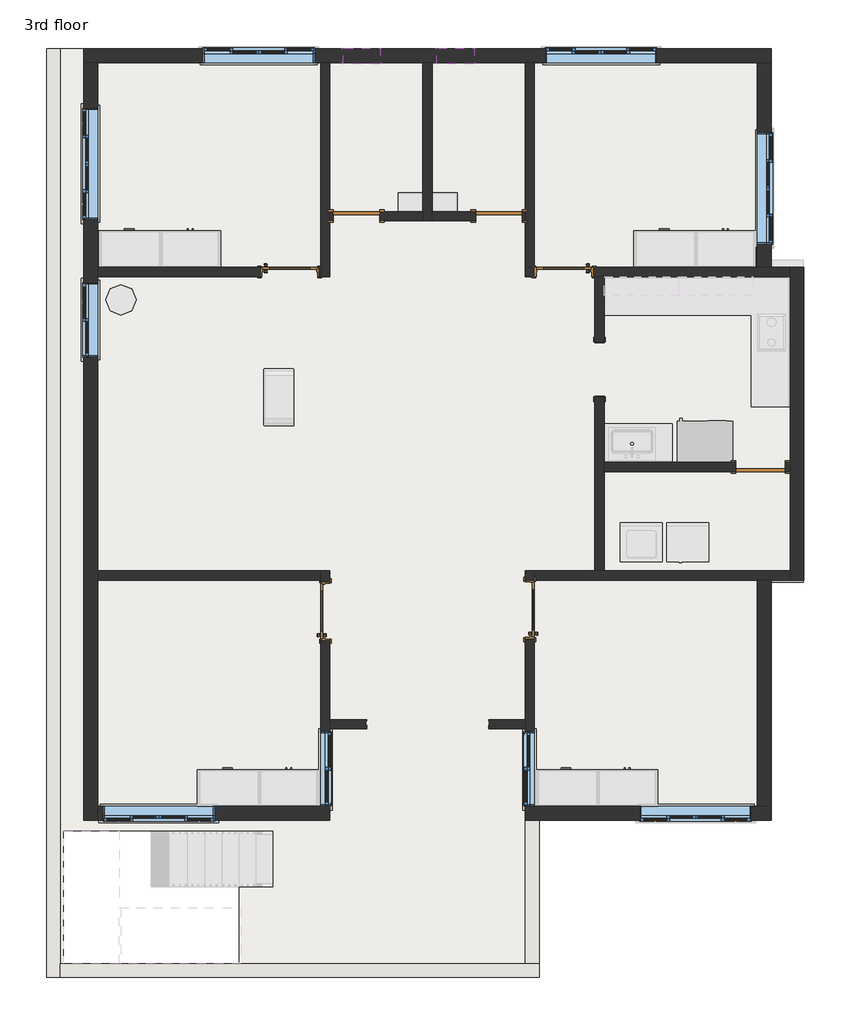
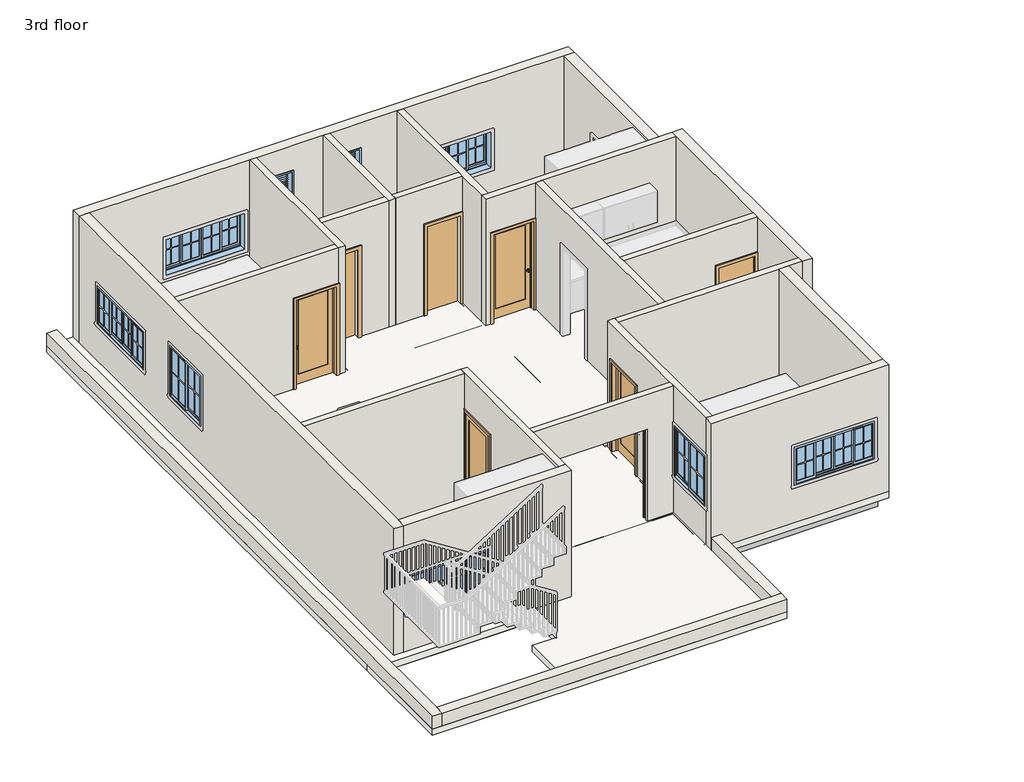
# One storey, part 1 of 4: 24 walls, 11 windows, 7 beams, 7 doors, 1 slab.
"""IFC4 building model written with IfcOpenShell, lengths in millimetres."""

from ifc_helpers import new_model, si_unit, frame, origin, place, context, project, spatial, polyline, outline, extrude, faceted_brep, transform, mapped, element, save
from components import door_010cc4d9, door_5a860750, door_e2b13fe9, door_a9addea7, door_bb092f7c, window_f2d8fef0, window_c1e3dfc0, window_49fe3060, window_58cce754

model = new_model("IFC4")

# Units and contexts
model_context = context("Model", 3, world=origin())
ifc_project = project(units=[si_unit("LENGTHUNIT", "METRE", prefix="MILLI")], contexts=[model_context])

# Site, building, storey
site = spatial("IfcSite", under=ifc_project)
building = spatial("IfcBuilding", under=site)
storey = spatial("IfcBuildingStorey", under=building, Name="3rd floor", Elevation=10210.8)

# Beams
placement = place(None, origin())
element("IfcBeam", 1, ObjectType="Concrete-Rectangular Beam", at=placement, inside=storey, context=model_context, shape_type="SweptSolid", body=[
    extrude(outline(polyline([(-1593.2124084, 1316.1961804), (-1364.6124084, 1316.1961804), (-1364.6124084, -2163.6038196), (-1593.2124084, -2163.6038196), (-1593.2124084, 1316.1961804)])), frame((0.0, 0.0, 9906.0), z_axis=(0.0, 0.0, 1.0), x_axis=(1.0, 0.0, 0.0)), (0.0, 0.0, 1.0), 304.8),
])
element("IfcBeam", 2, ObjectType="Concrete-Rectangular Beam", at=placement, inside=storey, context=model_context, shape_type="Brep", body=[
    faceted_brep([(-1593.2124084, -2201.7038196, 10210.8), (-5212.7124084, -2201.7038196, 10210.8), (-5441.3124084, -2201.7038196, 10210.8), (-5441.3124084, -2239.8038196, 10210.8), (-5174.6124084, -2239.8038196, 10210.8), (-5174.6124084, -2430.3038196, 10210.8), (-1593.2124084, -2430.3038196, 10210.8), (-1593.2124084, -2201.7038196, 9906.0), (-5212.7124084, -2201.7038196, 9906.0), (-5441.3124084, -2201.7038196, 9906.0), (-1593.2124084, -2430.3038196, 9906.0), (-5174.6124084, -2430.3038196, 9906.0), (-5174.6124084, -2239.8038196, 9906.0), (-5441.3124084, -2239.8038196, 9906.0)], [[[0, 1, 2, 3, 4, 5, 6]], [[0, 7, 8, 9, 2, 1]], [[9, 8, 7, 10, 11, 12, 13]], [[10, 6, 5, 11]], [[7, 0, 6, 10]], [[2, 9, 13, 3]], [[12, 4, 3, 13]], [[4, 12, 11, 5]]]),
])
element("IfcBeam", 3, ObjectType="Concrete-Rectangular Beam", at=placement, inside=storey, context=model_context, shape_type="Brep", body=[
    faceted_brep([(-8756.0124084, -2468.4038196, 10210.8), (-8756.0124084, -2239.8038196, 10210.8), (-8794.1124084, -2239.8038196, 10210.8), (-12413.6124084, -2239.8038196, 10210.8), (-12413.6124084, -2468.4038196, 10210.8), (-8756.0124084, -2239.8038196, 9906.0), (-8794.1124084, -2239.8038196, 9906.0), (-12413.6124084, -2239.8038196, 9906.0), (-8756.0124084, -2468.4038196, 9906.0), (-12413.6124084, -2468.4038196, 9906.0)], [[[0, 1, 2, 3, 4]], [[1, 5, 6, 7, 3, 2]], [[5, 8, 9, 7, 6]], [[8, 0, 4, 9]], [[1, 0, 8, 5]], [[4, 3, 7, 9]]]),
])
element("IfcBeam", 4, ObjectType="Concrete-Rectangular Beam", at=placement, inside=storey, context=model_context, shape_type="SweptSolid", body=[
    extrude(outline(polyline([(-12642.2124084, 9875.9961804), (-12413.6124084, 9875.9961804), (-12413.6124084, 6751.7961804), (-12642.2124084, 6751.7961804), (-12642.2124084, 9875.9961804)])), frame((0.0, 0.0, 9906.0), z_axis=(0.0, 0.0, 1.0), x_axis=(1.0, 0.0, 0.0)), (0.0, 0.0, 1.0), 304.8),
    extrude(outline(polyline([(-12413.6124084, -2163.6038196), (-12642.2124084, -2163.6038196), (-12642.2124084, 1392.3961804), (-12413.6124084, 1392.3961804), (-12413.6124084, -2163.6038196)])), frame((0.0, 0.0, 9906.0), z_axis=(0.0, 0.0, 1.0), x_axis=(1.0, 0.0, 0.0)), (0.0, 0.0, 1.0), 304.8),
    extrude(outline(polyline([(-12413.6124084, 1697.1961804), (-12642.2124084, 1697.1961804), (-12642.2124084, 6446.9961804), (-12413.6124084, 6446.9961804), (-12413.6124084, 1697.1961804)])), frame((0.0, 0.0, 9906.0), z_axis=(0.0, 0.0, 1.0), x_axis=(1.0, 0.0, 0.0)), (0.0, 0.0, 1.0), 304.8),
])
element("IfcBeam", 5, ObjectType="Concrete-Rectangular Beam", at=placement, inside=storey, context=model_context, shape_type="Brep", body=[
    faceted_brep([(-843.9124084, 1659.0961804, 10210.8), (-843.9124084, 1430.4961804, 10210.8), (-843.9124084, 1430.4961804, 9906.0), (-843.9124084, 1659.0961804, 9906.0), (-5098.4124084, 1659.0961804, 10210.8), (-5098.4124084, 1468.5961804, 10210.8), (-5403.2124084, 1468.5961804, 10210.8), (-5403.2124084, 1659.0961804, 10210.8), (-5441.3124084, 1659.0961804, 10210.8), (-8565.5124084, 1659.0961804, 10210.8), (-8603.6124084, 1659.0961804, 10210.8), (-8603.6124084, 1468.5961804, 10210.8), (-8908.4124084, 1468.5961804, 10210.8), (-8908.4124084, 1659.0961804, 10210.8), (-12413.6124084, 1659.0961804, 10210.8), (-12413.6124084, 1430.4961804, 10210.8), (-8794.1124084, 1430.4961804, 10210.8), (-8565.5124084, 1430.4961804, 10210.8), (-5441.3124084, 1430.4961804, 10210.8), (-5212.7124084, 1430.4961804, 10210.8), (-1593.2124084, 1430.4961804, 10210.8), (-1593.2124084, 1620.9961804, 10210.8), (-1364.6124084, 1620.9961804, 10210.8), (-1364.6124084, 1430.4961804, 10210.8), (-1364.6124084, 1430.4961804, 9906.0), (-1364.6124084, 1620.9961804, 9906.0), (-1593.2124084, 1620.9961804, 9906.0), (-1593.2124084, 1430.4961804, 9906.0), (-5212.7124084, 1430.4961804, 9906.0), (-5441.3124084, 1430.4961804, 9906.0), (-8565.5124084, 1430.4961804, 9906.0), (-8794.1124084, 1430.4961804, 9906.0), (-12413.6124084, 1430.4961804, 9906.0), (-12413.6124084, 1659.0961804, 9906.0), (-8908.4124084, 1659.0961804, 9906.0), (-8908.4124084, 1468.5961804, 9906.0), (-8603.6124084, 1468.5961804, 9906.0), (-8603.6124084, 1659.0961804, 9906.0), (-8565.5124084, 1659.0961804, 9906.0), (-5441.3124084, 1659.0961804, 9906.0), (-5403.2124084, 1659.0961804, 9906.0), (-5403.2124084, 1468.5961804, 9906.0), (-5098.4124084, 1468.5961804, 9906.0), (-5098.4124084, 1659.0961804, 9906.0)], [[[0, 1, 2, 3]], [[1, 0, 4, 5, 6, 7, 8, 9, 10, 11, 12, 13, 14, 15, 16, 17, 18, 19, 20, 21, 22, 23]], [[2, 1, 23, 24]], [[3, 2, 24, 25, 26, 27, 28, 29, 30, 31, 32, 33, 34, 35, 36, 37, 38, 39, 40, 41, 42, 43]], [[0, 3, 43, 4]], [[15, 14, 33, 32]], [[23, 22, 25, 24]], [[21, 20, 27, 26]], [[22, 21, 26, 25]], [[15, 32, 31, 30, 29, 28, 27, 20, 19, 18, 17, 16]], [[11, 10, 37, 36]], [[12, 11, 36, 35]], [[13, 12, 35, 34]], [[33, 14, 13, 34]], [[42, 5, 4, 43]], [[5, 42, 41, 6]], [[6, 41, 40, 7]], [[37, 10, 9, 8, 7, 40, 39, 38]]]),
])
element("IfcBeam", 6, ObjectType="Concrete-Rectangular Beam", at=placement, inside=storey, context=model_context, shape_type="Brep", body=[
    faceted_brep([(-8794.1124084, -2239.8038196, 10210.8), (-8756.0124084, -2239.8038196, 10210.8), (-8565.5124084, -2239.8038196, 10210.8), (-8565.5124084, -1007.9038196, 10210.8), (-8565.5124084, -779.3038196, 10210.8), (-8565.5124084, 1430.4961804, 10210.8), (-8794.1124084, 1430.4961804, 10210.8), (-8794.1124084, -2239.8038196, 9906.0), (-8794.1124084, 1430.4961804, 9906.0), (-8565.5124084, -2239.8038196, 9906.0), (-8756.0124084, -2239.8038196, 9906.0), (-8565.5124084, 1430.4961804, 9906.0), (-8565.5124084, -779.3038196, 9906.0), (-8565.5124084, -1007.9038196, 9906.0)], [[[0, 1, 2, 3, 4, 5, 6]], [[7, 0, 6, 8]], [[9, 10, 7, 8, 11, 12, 13]], [[11, 5, 4, 3, 2, 9, 13, 12]], [[2, 1, 0, 7, 10, 9]], [[5, 11, 8, 6]]]),
    faceted_brep([(-8794.1124084, 9914.0961804, 10210.8), (-8565.5124084, 9914.0961804, 10210.8), (-8565.5124084, 9914.0961804, 9906.0), (-8794.1124084, 9914.0961804, 9906.0), (-8794.1124084, 6713.6961804, 10210.8), (-8794.1124084, 6713.6961804, 9906.0), (-8756.0124084, 6713.6961804, 9906.0), (-8756.0124084, 6713.6961804, 10210.8), (-8756.0124084, 6751.7961804, 10210.8), (-8565.5124084, 6751.7961804, 10210.8), (-8565.5124084, 7323.2961804, 10210.8), (-8565.5124084, 7551.8961804, 10210.8), (-8565.5124084, 7551.8961804, 9906.0), (-8565.5124084, 7323.2961804, 9906.0), (-8565.5124084, 6751.7961804, 9906.0), (-8756.0124084, 6751.7961804, 9906.0)], [[[0, 1, 2, 3]], [[4, 5, 6, 7]], [[1, 0, 4, 7, 8, 9, 10, 11]], [[3, 2, 12, 13, 14, 15, 6, 5]], [[0, 3, 5, 4]], [[2, 1, 11, 10, 9, 14, 13, 12]], [[7, 6, 15, 8]], [[9, 8, 15, 14]]]),
    faceted_brep([(-8794.1124084, 6485.0961804, 9906.0), (-8794.1124084, 6485.0961804, 10210.8), (-8756.0124084, 6485.0961804, 10210.8), (-8756.0124084, 6485.0961804, 9906.0), (-8565.5124084, 1659.0961804, 9906.0), (-8565.5124084, 1659.0961804, 10210.8), (-8603.6124084, 1659.0961804, 10210.8), (-8603.6124084, 1659.0961804, 9906.0), (-8565.5124084, 6446.9961804, 9906.0), (-8565.5124084, 6446.9961804, 10210.8), (-8794.1124084, 1697.1961804, 10210.8), (-8603.6124084, 1697.1961804, 10210.8), (-8756.0124084, 6446.9961804, 10210.8), (-8794.1124084, 1697.1961804, 9906.0), (-8603.6124084, 1697.1961804, 9906.0), (-8756.0124084, 6446.9961804, 9906.0)], [[[0, 1, 2, 3]], [[4, 5, 6, 7]], [[5, 4, 8, 9]], [[2, 1, 10, 11, 6, 5, 9, 12]], [[1, 0, 13, 10]], [[8, 4, 7, 14, 13, 0, 3, 15]], [[9, 8, 15, 12]], [[3, 2, 12, 15]], [[14, 11, 10, 13]], [[11, 14, 7, 6]]]),
])
element("IfcBeam", 7, ObjectType="Concrete-Rectangular Beam", at=placement, inside=storey, context=model_context, shape_type="SweptSolid", body=[
    extrude(outline(polyline([(-5441.3124084, -779.3038196), (-5441.3124084, -1007.9038196), (-8565.5124084, -1007.9038196), (-8565.5124084, -779.3038196), (-5441.3124084, -779.3038196)])), frame((0.0, 0.0, 9906.0), z_axis=(0.0, 0.0, 1.0), x_axis=(1.0, 0.0, 0.0)), (0.0, 0.0, 1.0), 304.8),
])

# Doors
door_shape = door_010cc4d9(model_context)
element("IfcDoor", 8, ObjectType="Door-Interior-Single-1_Panel-Wood : 36\" x 84\"", at=placement, inside=storey, context=model_context, shape_type="MappedRepresentation", body=[
    mapped(door_shape, transform((-9264.0124084, 6526.3711804, 10210.8), x_axis=(1.0, 0.0, 0.0), y_axis=(0.0, 1.0, 0.0), z_axis=(0.0, 0.0, 1.0))),
])
element("IfcDoor", 9, ObjectType="Door-Interior-Single-1_Panel-Wood : 36\" x 84\"", at=placement, inside=storey, context=model_context, shape_type="MappedRepresentation", body=[
    mapped(door_shape, transform((-8682.9874084, 960.5961804, 10210.8), x_axis=(0.0, 1.0, 0.0), y_axis=(-1.0, 0.0, 0.0), z_axis=(0.0, 0.0, 1.0))),
])
door_2_shape = door_5a860750(model_context)
element("IfcDoor", 10, ObjectType="Door-Interior-Single-1_Panel-Wood : 36\" x 84\"", at=placement, inside=storey, context=model_context, shape_type="MappedRepresentation", body=[
    mapped(door_2_shape, transform((-4768.2124084, 6526.3711804, 10210.8), x_axis=(-1.0, 0.0, 0.0), y_axis=(0.0, -1.0, 0.0), z_axis=(0.0, 0.0, 1.0))),
])
element("IfcDoor", 11, ObjectType="Door-Interior-Single-1_Panel-Wood : 36\" x 84\"", at=placement, inside=storey, context=model_context, shape_type="MappedRepresentation", body=[
    mapped(door_2_shape, transform((-5323.8374084, 985.9961804, 10210.8), x_axis=(0.0, 1.0, 0.0), y_axis=(-1.0, 0.0, 0.0), z_axis=(0.0, 0.0, 1.0))),
])
door_3_shape = door_e2b13fe9(model_context)
element("IfcDoor", 12, ObjectType="Single-Flush : 30\" x 84\"", at=placement, inside=storey, context=model_context, shape_type="MappedRepresentation", body=[
    mapped(door_3_shape, transform((-8171.8124084, 7437.5961804, 10210.8), x_axis=(-1.0, 0.0, 0.0), y_axis=(0.0, -1.0, 0.0), z_axis=(0.0, 0.0, 1.0))),
])
door_4_shape = door_a9addea7(model_context)
element("IfcDoor", 13, ObjectType="Single-Flush : 30\" x 84\"", at=placement, inside=storey, context=model_context, shape_type="MappedRepresentation", body=[
    mapped(door_4_shape, transform((-5835.0124084, 7437.5961804, 10210.8), x_axis=(1.0, 0.0, 0.0), y_axis=(0.0, 1.0, 0.0), z_axis=(0.0, 0.0, 1.0))),
])
door_5_shape = door_bb092f7c(model_context)
element("IfcDoor", 14, ObjectType="Single-Flush : 32\" x 84\"", at=placement, inside=storey, context=model_context, shape_type="MappedRepresentation", body=[
    mapped(door_5_shape, transform((-1542.4124084, 3322.7961804, 10210.8), x_axis=(1.0, 0.0, 0.0), y_axis=(0.0, 1.0, 0.0), z_axis=(0.0, 0.0, 1.0))),
])

# Slab
element("IfcSlab", 15, ObjectType="Generic - 6\"", at=placement, inside=storey, context=model_context, shape_type="SweptSolid", body=[
    extrude(outline(polyline([(-1364.6124084, 10180.7961804), (-1364.6124084, 6599.3961804), (-831.2124084, 6599.3961804), (-831.2124084, 1468.5961804), (-1364.6124084, 1468.5961804), (-1364.6124084, -2468.4038196), (-5174.6124084, -2468.4038196), (-5174.6124084, -5046.5038196), (-13251.8124084, -5046.5038196), (-13251.8124084, -2468.4038196), (-13251.8124084, 10180.7961804), (-1364.6124084, 10180.7961804)]), holes=[polyline([(-9543.8120641, -3536.9669819), (-9543.8120641, -2647.9669819), (-12972.8120641, -2647.9669819), (-12972.8120641, -4817.9038196), (-10102.6120641, -4817.9038196), (-10102.6120641, -3536.9669819), (-9543.8120641, -3536.9669819)])]), frame((0.0, 0.0, 10058.4), z_axis=(0.0, 0.0, 1.0), x_axis=(1.0, 0.0, 0.0)), (0.0, 0.0, 1.0), 152.4),
])

# Walls
element("IfcWall", 16, ObjectType="Generic - 6\"", at=placement, inside=storey, context=model_context, shape_type="Brep", body=[
    faceted_brep([(-8756.0124084, 9952.1961804, 10210.8), (-8756.0124084, 6599.3961804, 10210.8), (-8756.0124084, 6446.9961804, 10210.8), (-8756.0124084, 6446.9961804, 13258.8), (-8756.0124084, 6599.3961804, 13258.8), (-8756.0124084, 9952.1961804, 13258.8), (-8603.6124084, 9952.1961804, 10210.8), (-8603.6124084, 9952.1961804, 13258.8), (-8603.6124084, 7513.7961804, 13258.8), (-8603.6124084, 7361.3961804, 13258.8), (-8603.6124084, 6446.9961804, 13258.8), (-8603.6124084, 6446.9961804, 10210.8), (-8603.6124084, 7361.3961804, 10210.8), (-8603.6124084, 7513.7961804, 10210.8)], [[[0, 1, 2, 3, 4, 5]], [[6, 7, 8, 9, 10, 11, 12, 13]], [[2, 1, 0, 6, 13, 12, 11]], [[0, 5, 7, 6]], [[3, 2, 11, 10]], [[5, 4, 3, 10, 9, 8, 7]]]),
])
element("IfcWall", 17, ObjectType="Generic - 6\"", at=placement, inside=storey, context=model_context, shape_type="SweptSolid", body=[
    extrude(outline(polyline([(10210.8, -8756.0124084), (13258.8, -8756.0124084), (13258.8, -12413.6124084), (10210.8, -12413.6124084), (10210.8, -9746.6124084), (12369.8, -9746.6124084), (12369.8, -8781.4124084), (10210.8, -8781.4124084), (10210.8, -8756.0124084)])), frame((0.0, 6446.9961804, 0.0), z_axis=(0.0, 1.0, 0.0), x_axis=(0.0, 0.0, 1.0)), (0.0, 0.0, 1.0), 152.4),
])
element("IfcWall", 18, ObjectType="Generic - 6\"", at=placement, inside=storey, context=model_context, shape_type="Brep", body=[
    faceted_brep([(-7079.6124084, 9952.1961804, 10210.8), (-7079.6124084, 7513.7961804, 10210.8), (-7079.6124084, 7361.3961804, 10210.8), (-7079.6124084, 7361.3961804, 13258.8), (-7079.6124084, 7513.7961804, 13258.8), (-7079.6124084, 9952.1961804, 13258.8), (-6927.2124084, 9952.1961804, 10210.8), (-6927.2124084, 9952.1961804, 13258.8), (-6927.2124084, 7513.7961804, 13258.8), (-6927.2124084, 7361.3961804, 13258.8), (-6927.2124084, 7361.3961804, 10210.8), (-6927.2124084, 7513.7961804, 10210.8)], [[[0, 1, 2, 3, 4, 5]], [[6, 7, 8, 9, 10, 11]], [[2, 1, 0, 6, 11, 10]], [[0, 5, 7, 6]], [[3, 2, 10, 9]], [[5, 4, 3, 9, 8, 7]]]),
])
element("IfcWall", 19, ObjectType="Generic - 6\"", at=placement, inside=storey, context=model_context, shape_type="SweptSolid", body=[
    extrude(outline(polyline([(10210.8, -7079.6124084), (13258.8, -7079.6124084), (13258.8, -8603.6124084), (10210.8, -8603.6124084), (10210.8, -8552.8124084), (12344.4, -8552.8124084), (12344.4, -7790.8124084), (10210.8, -7790.8124084), (10210.8, -7079.6124084)])), frame((0.0, 7361.3961804, 0.0), z_axis=(0.0, 1.0, 0.0), x_axis=(0.0, 0.0, 1.0)), (0.0, 0.0, 1.0), 152.4),
])
element("IfcWall", 20, ObjectType="Generic - 6\"", at=placement, inside=storey, context=model_context, shape_type="SweptSolid", body=[
    extrude(outline(polyline([(13258.8, -6927.2124084), (10210.8, -6927.2124084), (10210.8, -6216.0124084), (12344.4, -6216.0124084), (12344.4, -5454.0124084), (10210.8, -5454.0124084), (10210.8, -5403.2124084), (13258.8, -5403.2124084), (13258.8, -6927.2124084)])), frame((0.0, 7361.3961804, 0.0), z_axis=(0.0, 1.0, 0.0), x_axis=(0.0, 0.0, 1.0)), (0.0, 0.0, 1.0), 152.4),
])
element("IfcWall", 21, ObjectType="Generic - 6\"", at=placement, inside=storey, context=model_context, shape_type="Brep", body=[
    faceted_brep([(-5250.8124084, 6599.3961804, 10210.8), (-5250.8124084, 9952.1961804, 10210.8), (-5250.8124084, 9952.1961804, 13258.8), (-5250.8124084, 6599.3961804, 13258.8), (-5403.2124084, 6599.3961804, 10210.8), (-5403.2124084, 6599.3961804, 13258.8), (-5403.2124084, 7361.3961804, 13258.8), (-5403.2124084, 7513.7961804, 13258.8), (-5403.2124084, 9952.1961804, 13258.8), (-5403.2124084, 9952.1961804, 10210.8), (-5403.2124084, 7513.7961804, 10210.8), (-5403.2124084, 7361.3961804, 10210.8)], [[[0, 1, 2, 3]], [[4, 5, 6, 7, 8, 9, 10, 11]], [[1, 0, 4, 11, 10, 9]], [[2, 1, 9, 8]], [[0, 3, 5, 4]], [[3, 2, 8, 7, 6, 5]]]),
])
element("IfcWall", 22, ObjectType="Generic - 6\"", at=placement, inside=storey, context=model_context, shape_type="Brep", body=[
    faceted_brep([(-5403.2124084, 6599.3961804, 10210.8), (-5403.2124084, 6599.3961804, 13258.8), (-5250.8124084, 6599.3961804, 13258.8), (-1593.2124084, 6599.3961804, 13258.8), (-1364.6124084, 6599.3961804, 13258.8), (-1059.8124084, 6599.3961804, 13258.8), (-1059.8124084, 6599.3961804, 10210.8), (-1364.6124084, 6599.3961804, 10210.8), (-1593.2124084, 6599.3961804, 10210.8), (-4285.6124084, 6599.3961804, 10210.8), (-4285.6124084, 6599.3961804, 12369.8), (-5250.8124084, 6599.3961804, 12369.8), (-5250.8124084, 6599.3961804, 10210.8), (-1059.8124084, 6446.9961804, 13258.8), (-4107.8124084, 6446.9961804, 13258.8), (-4260.2124084, 6446.9961804, 13258.8), (-5403.2124084, 6446.9961804, 13258.8), (-5403.2124084, 6446.9961804, 10210.8), (-5250.8124084, 6446.9961804, 10210.8), (-5250.8124084, 6446.9961804, 12369.8), (-4285.6124084, 6446.9961804, 12369.8), (-4285.6124084, 6446.9961804, 10210.8), (-4260.2124084, 6446.9961804, 10210.8), (-4107.8124084, 6446.9961804, 10210.8), (-1059.8124084, 6446.9961804, 10210.8)], [[[0, 1, 2, 3, 4, 5, 6, 7, 8, 9, 10, 11, 12]], [[13, 14, 15, 16, 17, 18, 19, 20, 21, 22, 23, 24]], [[17, 0, 12, 18]], [[6, 24, 23, 22, 21, 9, 8, 7]], [[1, 0, 17, 16]], [[6, 5, 13, 24]], [[11, 19, 18, 12]], [[19, 11, 10, 20]], [[20, 10, 9, 21]], [[16, 15, 14, 13, 5, 4, 3, 2, 1]]]),
])
element("IfcWall", 23, ObjectType="Generic - 6\"", at=placement, inside=storey, context=model_context, shape_type="SweptSolid", body=[
    extrude(outline(polyline([(-8756.0124084, 1468.5961804), (-12413.6124084, 1468.5961804), (-12413.6124084, 1620.9961804), (-8756.0124084, 1620.9961804), (-8756.0124084, 1468.5961804)])), frame((0.0, 0.0, 10210.8), z_axis=(0.0, 0.0, 1.0), x_axis=(1.0, 0.0, 0.0)), (0.0, 0.0, 1.0), 3048.0),
])
element("IfcWall", 24, ObjectType="Generic - 6\"", at=placement, inside=storey, context=model_context, shape_type="Brep", body=[
    faceted_brep([(-5403.2124084, -2239.8038196, 10210.8), (-5403.2124084, -2239.8038196, 13258.8), (-5403.2124084, -969.8038196, 13258.8), (-5403.2124084, -817.4038196, 13258.8), (-5403.2124084, 1620.9961804, 13258.8), (-5403.2124084, 1620.9961804, 10210.8), (-5403.2124084, 1468.5961804, 10210.8), (-5403.2124084, 1468.5961804, 12369.8), (-5403.2124084, 503.3961804, 12369.8), (-5403.2124084, 503.3961804, 10210.8), (-5403.2124084, -817.4038196, 10210.8), (-5403.2124084, -969.8038196, 10210.8), (-5403.2124084, -1014.2538196, 11125.2), (-5403.2124084, -1014.2538196, 12344.4), (-5403.2124084, -2233.4538196, 12344.4), (-5403.2124084, -2233.4538196, 11125.2), (-5250.8124084, -2239.8038196, 13258.8), (-5250.8124084, -2239.8038196, 10210.8), (-5250.8124084, 503.3961804, 10210.8), (-5250.8124084, 503.3961804, 12369.8), (-5250.8124084, 1468.5961804, 12369.8), (-5250.8124084, 1468.5961804, 10210.8), (-5250.8124084, 1620.9961804, 10210.8), (-5250.8124084, 1620.9961804, 13258.8), (-5250.8124084, 1468.5961804, 13258.8), (-5250.8124084, -1014.2538196, 12344.4), (-5250.8124084, -1014.2538196, 11125.2), (-5250.8124084, -2233.4538196, 11125.2), (-5250.8124084, -2233.4538196, 12344.4)], [[[0, 1, 2, 3, 4, 5, 6, 7, 8, 9, 10, 11], [12, 13, 14, 15]], [[16, 17, 18, 19, 20, 21, 22, 23, 24], [25, 26, 27, 28]], [[17, 0, 11, 10, 9, 18]], [[5, 22, 21, 6]], [[1, 0, 17, 16]], [[5, 4, 23, 22]], [[20, 7, 6, 21]], [[7, 20, 19, 8]], [[8, 19, 18, 9]], [[25, 13, 12, 26]], [[26, 12, 15, 27]], [[27, 15, 14, 28]], [[13, 25, 28, 14]], [[4, 3, 2, 1, 16, 24, 23]]]),
])
element("IfcWall", 25, ObjectType="Generic - 6\"", at=placement, inside=storey, context=model_context, shape_type="Brep", body=[
    faceted_brep([(-8756.0124084, 1620.9961804, 10210.8), (-8756.0124084, 1468.5961804, 10210.8), (-8756.0124084, 1443.1961804, 10210.8), (-8756.0124084, 1443.1961804, 12369.8), (-8756.0124084, 477.9961804, 12369.8), (-8756.0124084, 477.9961804, 10210.8), (-8756.0124084, -2239.8038196, 10210.8), (-8756.0124084, -2239.8038196, 13258.8), (-8756.0124084, 1468.5961804, 13258.8), (-8756.0124084, 1620.9961804, 13258.8), (-8756.0124084, -2233.4538196, 12344.4), (-8756.0124084, -2233.4538196, 11125.2), (-8756.0124084, -1014.2538196, 11125.2), (-8756.0124084, -1014.2538196, 12344.4), (-8603.6124084, 1443.1961804, 10210.8), (-8603.6124084, 1620.9961804, 10210.8), (-8603.6124084, 1620.9961804, 13258.8), (-8603.6124084, -817.4038196, 13258.8), (-8603.6124084, -969.8038196, 13258.8), (-8603.6124084, -2239.8038196, 13258.8), (-8603.6124084, -2239.8038196, 10210.8), (-8603.6124084, -969.8038196, 10210.8), (-8603.6124084, -817.4038196, 10210.8), (-8603.6124084, 477.9961804, 10210.8), (-8603.6124084, 477.9961804, 12369.8), (-8603.6124084, 1443.1961804, 12369.8), (-8603.6124084, -2233.4538196, 11125.2), (-8603.6124084, -2233.4538196, 12344.4), (-8603.6124084, -1014.2538196, 12344.4), (-8603.6124084, -1014.2538196, 11125.2)], [[[0, 1, 2, 3, 4, 5, 6, 7, 8, 9], [10, 11, 12, 13]], [[14, 15, 16, 17, 18, 19, 20, 21, 22, 23, 24, 25], [26, 27, 28, 29]], [[6, 5, 23, 22, 21, 20]], [[2, 1, 0, 15, 14]], [[25, 3, 2, 14]], [[3, 25, 24, 4]], [[4, 24, 23, 5]], [[0, 9, 16, 15]], [[10, 27, 26, 11]], [[11, 26, 29, 12]], [[12, 29, 28, 13]], [[27, 10, 13, 28]], [[9, 8, 7, 19, 18, 17, 16]], [[7, 6, 20, 19]]]),
])
element("IfcWall", 26, ObjectType="Generic - 6\"", at=placement, inside=storey, context=model_context, shape_type="Brep", body=[
    faceted_brep([(-4260.2124084, 6446.9961804, 13258.8), (-4260.2124084, 6446.9961804, 10210.8), (-4260.2124084, 5380.1961804, 10210.8), (-4260.2124084, 5380.1961804, 12344.4), (-4260.2124084, 4465.7961804, 12344.4), (-4260.2124084, 4465.7961804, 10210.8), (-4260.2124084, 1620.9961804, 10210.8), (-4260.2124084, 1620.9961804, 13258.8), (-4107.8124084, 6446.9961804, 10210.8), (-4107.8124084, 6446.9961804, 13258.8), (-4107.8124084, 3398.9961804, 13258.8), (-4107.8124084, 3246.5961804, 13258.8), (-4107.8124084, 1620.9961804, 13258.8), (-4107.8124084, 1620.9961804, 10210.8), (-4107.8124084, 3246.5961804, 10210.8), (-4107.8124084, 3398.9961804, 10210.8), (-4107.8124084, 4465.7961804, 10210.8), (-4107.8124084, 4465.7961804, 12344.4), (-4107.8124084, 5380.1961804, 12344.4), (-4107.8124084, 5380.1961804, 10210.8)], [[[0, 1, 2, 3, 4, 5, 6, 7]], [[8, 9, 10, 11, 12, 13, 14, 15, 16, 17, 18, 19]], [[1, 8, 19, 2]], [[13, 6, 5, 16, 15, 14]], [[1, 0, 9, 8]], [[7, 6, 13, 12]], [[4, 17, 16, 5]], [[18, 3, 2, 19]], [[17, 4, 3, 18]], [[0, 7, 12, 11, 10, 9]]]),
])
element("IfcWall", 27, ObjectType="Generic - 6\"", at=placement, inside=storey, context=model_context, shape_type="SweptSolid", body=[
    extrude(outline(polyline([(13258.8, -4107.8124084), (10210.8, -4107.8124084), (10210.8, -1948.8124084), (12344.4, -1948.8124084), (12344.4, -1136.0124084), (10210.8, -1136.0124084), (10210.8, -1059.8124084), (13258.8, -1059.8124084), (13258.8, -4107.8124084)])), frame((0.0, 3246.5961804, 0.0), z_axis=(0.0, 1.0, 0.0), x_axis=(0.0, 0.0, 1.0)), (0.0, 0.0, 1.0), 152.4),
])
element("IfcWall", 28, ObjectType="Generic - 6\"", at=placement, inside=storey, context=model_context, shape_type="Brep", body=[
    faceted_brep([(-5250.8124084, 1468.5961804, 10210.8), (-1593.2124084, 1468.5961804, 10210.8), (-1364.6124084, 1468.5961804, 10210.8), (-1059.8124084, 1468.5961804, 10210.8), (-1059.8124084, 1468.5961804, 13258.8), (-1364.6124084, 1468.5961804, 13258.8), (-1593.2124084, 1468.5961804, 13258.8), (-5250.8124084, 1468.5961804, 13258.8), (-5250.8124084, 1620.9961804, 10210.8), (-5250.8124084, 1620.9961804, 13258.8), (-4260.2124084, 1620.9961804, 13258.8), (-4107.8124084, 1620.9961804, 13258.8), (-1059.8124084, 1620.9961804, 13258.8), (-1059.8124084, 1620.9961804, 10210.8), (-4107.8124084, 1620.9961804, 10210.8), (-4260.2124084, 1620.9961804, 10210.8)], [[[0, 1, 2, 3, 4, 5, 6, 7]], [[8, 9, 10, 11, 12, 13, 14, 15]], [[3, 2, 1, 0, 8, 15, 14, 13]], [[4, 3, 13, 12]], [[0, 7, 9, 8]], [[7, 6, 5, 4, 12, 11, 10, 9]]]),
])
element("IfcWall", 29, ObjectType="Generic - 6\"", at=placement, inside=storey, context=model_context, shape_type="Brep", body=[
    faceted_brep([(-5403.2124084, -969.8038196, 10210.8), (-5403.2124084, -969.8038196, 13258.8), (-8603.6124084, -969.8038196, 13258.8), (-8603.6124084, -969.8038196, 10210.8), (-8003.4124084, -969.8038196, 10210.8), (-8003.4124084, -969.8038196, 12419.8), (-6003.4124084, -969.8038196, 12419.8), (-6003.4124084, -969.8038196, 10210.8), (-5403.2124084, -817.4038196, 13258.8), (-5403.2124084, -817.4038196, 10210.8), (-6003.4124084, -817.4038196, 10210.8), (-6003.4124084, -817.4038196, 12419.8), (-8003.4124084, -817.4038196, 12419.8), (-8003.4124084, -817.4038196, 10210.8), (-8603.6124084, -817.4038196, 10210.8), (-8603.6124084, -817.4038196, 13258.8), (-8003.4124084, -837.4038196, 10210.8), (-8018.4124084, -837.4038196, 10210.8), (-8018.4124084, -907.4038196, 10210.8), (-8003.4124084, -907.4038196, 10210.8), (-6003.4124084, -907.4038196, 10210.8), (-5988.4124084, -907.4038196, 10210.8), (-5988.4124084, -837.4038196, 10210.8), (-6003.4124084, -837.4038196, 10210.8), (-6003.4124084, -837.4038196, 12419.8), (-8003.4124084, -837.4038196, 12419.8), (-8003.4124084, -907.4038196, 12419.8), (-6003.4124084, -907.4038196, 12419.8), (-8018.4124084, -907.4038196, 12434.8), (-5988.4124084, -907.4038196, 12434.8), (-5988.4124084, -837.4038196, 12434.8), (-8018.4124084, -837.4038196, 12434.8)], [[[0, 1, 2, 3, 4, 5, 6, 7]], [[8, 9, 10, 11, 12, 13, 14, 15]], [[3, 14, 13, 16, 17, 18, 19, 4]], [[9, 0, 7, 20, 21, 22, 23, 10]], [[1, 0, 9, 8]], [[3, 2, 15, 14]], [[24, 25, 12, 11]], [[26, 27, 6, 5]], [[19, 26, 5, 4]], [[27, 20, 7, 6]], [[27, 26, 19, 18, 28, 29, 21, 20]], [[21, 29, 30, 22]], [[25, 24, 23, 22, 30, 31, 17, 16]], [[23, 24, 11, 10]], [[25, 16, 13, 12]], [[28, 18, 17, 31]], [[29, 28, 31, 30]], [[2, 1, 8, 15]]]),
])
element("IfcWall", 30, ObjectType="Generic - 9\"", at=placement, inside=storey, context=model_context, shape_type="Brep", body=[
    faceted_brep([(-12642.2124084, 9952.1961804, 10210.8), (-12413.6124084, 9952.1961804, 10210.8), (-8756.0124084, 9952.1961804, 10210.8), (-8603.6124084, 9952.1961804, 10210.8), (-7079.6124084, 9952.1961804, 10210.8), (-6927.2124084, 9952.1961804, 10210.8), (-5403.2124084, 9952.1961804, 10210.8), (-5250.8124084, 9952.1961804, 10210.8), (-1593.2124084, 9952.1961804, 10210.8), (-1364.6124084, 9952.1961804, 10210.8), (-1364.6124084, 9952.1961804, 13258.8), (-1593.2124084, 9952.1961804, 13258.8), (-5250.8124084, 9952.1961804, 13258.8), (-5403.2124084, 9952.1961804, 13258.8), (-6927.2124084, 9952.1961804, 13258.8), (-7079.6124084, 9952.1961804, 13258.8), (-8603.6124084, 9952.1961804, 13258.8), (-8756.0124084, 9952.1961804, 13258.8), (-12413.6124084, 9952.1961804, 13258.8), (-12642.2124084, 9952.1961804, 13258.8), (-3244.2124084, 9952.1961804, 12039.6), (-3244.2124084, 9952.1961804, 11125.2), (-5073.0124084, 9952.1961804, 11125.2), (-5073.0124084, 9952.1961804, 12039.6), (-8857.6124084, 9952.1961804, 12039.6), (-8857.6124084, 9952.1961804, 11125.2), (-10686.4124084, 9952.1961804, 11125.2), (-10686.4124084, 9952.1961804, 12039.6), (-8387.7124084, 9952.1961804, 12039.6), (-8387.7124084, 9952.1961804, 12649.2), (-7778.1124084, 9952.1961804, 12649.2), (-7778.1124084, 9952.1961804, 12039.6), (-6851.0124084, 9952.1961804, 12039.6), (-6851.0124084, 9952.1961804, 12649.2), (-6241.4124084, 9952.1961804, 12649.2), (-6241.4124084, 9952.1961804, 12039.6), (-1364.6124084, 10180.7961804, 10210.8), (-12642.2124084, 10180.7961804, 10210.8), (-12642.2124084, 10180.7961804, 13258.8), (-1364.6124084, 10180.7961804, 13258.8), (-3244.2124084, 10180.7961804, 11125.2), (-3244.2124084, 10180.7961804, 12039.6), (-5073.0124084, 10180.7961804, 12039.6), (-5073.0124084, 10180.7961804, 11125.2), (-8857.6124084, 10180.7961804, 11125.2), (-8857.6124084, 10180.7961804, 12039.6), (-10686.4124084, 10180.7961804, 12039.6), (-10686.4124084, 10180.7961804, 11125.2), (-8387.7124084, 10180.7961804, 12649.2), (-8387.7124084, 10180.7961804, 12039.6), (-7778.1124084, 10180.7961804, 12039.6), (-7778.1124084, 10180.7961804, 12649.2), (-6851.0124084, 10180.7961804, 12649.2), (-6851.0124084, 10180.7961804, 12039.6), (-6241.4124084, 10180.7961804, 12039.6), (-6241.4124084, 10180.7961804, 12649.2)], [[[0, 1, 2, 3, 4, 5, 6, 7, 8, 9, 10, 11, 12, 13, 14, 15, 16, 17, 18, 19], [20, 21, 22, 23], [24, 25, 26, 27], [28, 29, 30, 31], [32, 33, 34, 35]], [[36, 37, 38, 39], [40, 41, 42, 43], [44, 45, 46, 47], [48, 49, 50, 51], [52, 53, 54, 55]], [[9, 8, 7, 6, 5, 4, 3, 2, 1, 0, 37, 36]], [[0, 19, 38, 37]], [[10, 9, 36, 39]], [[20, 41, 40, 21]], [[21, 40, 43, 22]], [[22, 43, 42, 23]], [[41, 20, 23, 42]], [[24, 45, 44, 25]], [[25, 44, 47, 26]], [[46, 27, 26, 47]], [[45, 24, 27, 46]], [[49, 48, 29, 28]], [[50, 49, 28, 31]], [[51, 50, 31, 30]], [[48, 51, 30, 29]], [[53, 52, 33, 32]], [[54, 53, 32, 35]], [[55, 54, 35, 34]], [[52, 55, 34, 33]], [[19, 18, 17, 16, 15, 14, 13, 12, 11, 10, 39, 38]]]),
])
element("IfcWall", 31, ObjectType="Generic - 9\"", at=placement, inside=storey, context=model_context, shape_type="Brep", body=[
    faceted_brep([(-12642.2124084, 9952.1961804, 10210.8), (-12642.2124084, -2468.4038196, 10210.8), (-12642.2124084, -2468.4038196, 13258.8), (-12642.2124084, 9952.1961804, 13258.8), (-12642.2124084, 5126.1961804, 12344.4), (-12642.2124084, 5126.1961804, 11125.2), (-12642.2124084, 6345.3961804, 11125.2), (-12642.2124084, 6345.3961804, 12344.4), (-12642.2124084, 9209.2461804, 11125.2), (-12642.2124084, 9209.2461804, 12039.6), (-12642.2124084, 7380.4461804, 12039.6), (-12642.2124084, 7380.4461804, 11125.2), (-12413.6124084, -2468.4038196, 10210.8), (-12413.6124084, -2239.8038196, 10210.8), (-12413.6124084, 1468.5961804, 10210.8), (-12413.6124084, 1620.9961804, 10210.8), (-12413.6124084, 6446.9961804, 10210.8), (-12413.6124084, 6599.3961804, 10210.8), (-12413.6124084, 9952.1961804, 10210.8), (-12413.6124084, 9952.1961804, 13258.8), (-12413.6124084, 6599.3961804, 13258.8), (-12413.6124084, 6446.9961804, 13258.8), (-12413.6124084, 1620.9961804, 13258.8), (-12413.6124084, 1468.5961804, 13258.8), (-12413.6124084, -2239.8038196, 13258.8), (-12413.6124084, -2468.4038196, 13258.8), (-12413.6124084, 5126.1961804, 11125.2), (-12413.6124084, 5126.1961804, 12344.4), (-12413.6124084, 6345.3961804, 12344.4), (-12413.6124084, 6345.3961804, 11125.2), (-12413.6124084, 9209.2461804, 12039.6), (-12413.6124084, 9209.2461804, 11125.2), (-12413.6124084, 7380.4461804, 11125.2), (-12413.6124084, 7380.4461804, 12039.6)], [[[0, 1, 2, 3], [4, 5, 6, 7], [8, 9, 10, 11]], [[12, 13, 14, 15, 16, 17, 18, 19, 20, 21, 22, 23, 24, 25], [26, 27, 28, 29], [30, 31, 32, 33]], [[1, 0, 18, 17, 16, 15, 14, 13, 12]], [[0, 3, 19, 18]], [[2, 1, 12, 25]], [[4, 27, 26, 5]], [[5, 26, 29, 6]], [[6, 29, 28, 7]], [[30, 9, 8, 31]], [[31, 8, 11, 32]], [[10, 33, 32, 11]], [[9, 30, 33, 10]], [[27, 4, 7, 28]], [[3, 2, 25, 24, 23, 22, 21, 20, 19]]]),
])
element("IfcWall", 32, ObjectType="Generic - 9\"", at=placement, inside=storey, context=model_context, shape_type="SweptSolid", body=[
    extrude(outline(polyline([(9952.1961804, 10210.8), (6599.3961804, 10210.8), (6599.3961804, 13258.8), (9952.1961804, 13258.8), (9952.1961804, 10210.8)]), holes=[polyline([(6980.3961804, 12039.6), (6980.3961804, 11125.2), (8809.1961804, 11125.2), (8809.1961804, 12039.6), (6980.3961804, 12039.6)])]), frame((-1593.2124084, 0.0, 0.0), z_axis=(1.0, 0.0, 0.0), x_axis=(0.0, 1.0, 0.0)), (0.0, 0.0, 1.0), 228.6),
])
element("IfcWall", 33, ObjectType="Generic - 9\"", at=placement, inside=storey, context=model_context, shape_type="Brep", body=[
    faceted_brep([(-12413.6124084, -2468.4038196, 10210.8), (-8603.6124084, -2468.4038196, 10210.8), (-8603.6124084, -2468.4038196, 13258.8), (-12413.6124084, -2468.4038196, 13258.8), (-12324.7124084, -2468.4038196, 11125.2), (-12324.7124084, -2468.4038196, 12039.6), (-10495.9124084, -2468.4038196, 12039.6), (-10495.9124084, -2468.4038196, 11125.2), (-8603.6124084, -2239.8038196, 10210.8), (-8756.0124084, -2239.8038196, 10210.8), (-12413.6124084, -2239.8038196, 10210.8), (-12413.6124084, -2239.8038196, 13258.8), (-8756.0124084, -2239.8038196, 13258.8), (-8603.6124084, -2239.8038196, 13258.8), (-12324.7124084, -2239.8038196, 12039.6), (-12324.7124084, -2239.8038196, 11125.2), (-10495.9124084, -2239.8038196, 11125.2), (-10495.9124084, -2239.8038196, 12039.6)], [[[0, 1, 2, 3], [4, 5, 6, 7]], [[8, 9, 10, 11, 12, 13], [14, 15, 16, 17]], [[1, 0, 10, 9, 8]], [[0, 3, 11, 10]], [[14, 5, 4, 15]], [[15, 4, 7, 16]], [[16, 7, 6, 17]], [[5, 14, 17, 6]], [[3, 2, 13, 12, 11]], [[2, 1, 8, 13]]]),
])
element("IfcWall", 34, ObjectType="Generic - 9\"", at=placement, inside=storey, context=model_context, shape_type="SweptSolid", body=[
    extrude(outline(polyline([(-1593.2124084, -2239.8038196), (-1593.2124084, 1468.5961804), (-1364.6124084, 1468.5961804), (-1364.6124084, -2239.8038196), (-1593.2124084, -2239.8038196)])), frame((0.0, 0.0, 10210.8), z_axis=(0.0, 0.0, 1.0), x_axis=(1.0, 0.0, 0.0)), (0.0, 0.0, 1.0), 3048.0),
])
element("IfcWall", 35, ObjectType="Generic - 9\"", at=placement, inside=storey, context=model_context, shape_type="Brep", body=[
    faceted_brep([(-1059.8124084, 6599.3961804, 10210.8), (-1059.8124084, 6446.9961804, 10210.8), (-1059.8124084, 3398.9961804, 10210.8), (-1059.8124084, 3246.5961804, 10210.8), (-1059.8124084, 1620.9961804, 10210.8), (-1059.8124084, 1468.5961804, 10210.8), (-1059.8124084, 1468.5961804, 13258.8), (-1059.8124084, 1620.9961804, 13258.8), (-1059.8124084, 3246.5961804, 13258.8), (-1059.8124084, 3398.9961804, 13258.8), (-1059.8124084, 6446.9961804, 13258.8), (-1059.8124084, 6599.3961804, 13258.8), (-831.2124084, 6599.3961804, 10210.8), (-831.2124084, 6599.3961804, 13258.8), (-831.2124084, 1468.5961804, 13258.8), (-831.2124084, 1468.5961804, 10210.8)], [[[0, 1, 2, 3, 4, 5, 6, 7, 8, 9, 10, 11]], [[12, 13, 14, 15]], [[5, 4, 3, 2, 1, 0, 12, 15]], [[0, 11, 13, 12]], [[6, 5, 15, 14]], [[11, 10, 9, 8, 7, 6, 14, 13]]]),
])
element("IfcWall", 36, ObjectType="Generic - 9\"", at=placement, inside=storey, context=model_context, shape_type="Brep", body=[
    faceted_brep([(-5403.2124084, -2468.4038196, 10210.8), (-5174.6124084, -2468.4038196, 10210.8), (-1364.6124084, -2468.4038196, 10210.8), (-1364.6124084, -2468.4038196, 13258.8), (-5174.6124084, -2468.4038196, 13258.8), (-5403.2124084, -2468.4038196, 13258.8), (-5403.2124084, -2468.4038196, 10515.6), (-3523.6124084, -2468.4038196, 11125.2), (-3523.6124084, -2468.4038196, 12039.6), (-1694.8124084, -2468.4038196, 12039.6), (-1694.8124084, -2468.4038196, 11125.2), (-1364.6124084, -2239.8038196, 10210.8), (-1593.2124084, -2239.8038196, 10210.8), (-5250.8124084, -2239.8038196, 10210.8), (-5403.2124084, -2239.8038196, 10210.8), (-5403.2124084, -2239.8038196, 13258.8), (-5250.8124084, -2239.8038196, 13258.8), (-1593.2124084, -2239.8038196, 13258.8), (-1364.6124084, -2239.8038196, 13258.8), (-3523.6124084, -2239.8038196, 12039.6), (-3523.6124084, -2239.8038196, 11125.2), (-1694.8124084, -2239.8038196, 11125.2), (-1694.8124084, -2239.8038196, 12039.6)], [[[0, 1, 2, 3, 4, 5, 6], [7, 8, 9, 10]], [[11, 12, 13, 14, 15, 16, 17, 18], [19, 20, 21, 22]], [[2, 1, 0, 14, 13, 12, 11]], [[3, 2, 11, 18]], [[19, 8, 7, 20]], [[20, 7, 10, 21]], [[21, 10, 9, 22]], [[8, 19, 22, 9]], [[18, 17, 16, 15, 5, 4, 3]], [[0, 6, 5, 15, 14]]]),
])
element("IfcWall", 37, ObjectType="Generic - 9\"", at=placement, inside=storey, context=model_context, shape_type="Brep", body=[
    faceted_brep([(-13251.8124084, 10180.7961804, 10210.8), (-13251.8124084, -5046.5038196, 10210.8), (-13251.8124084, -5046.5038196, 10515.6), (-13251.8124084, 10180.7961804, 10515.6), (-13023.2124084, 10180.7961804, 10210.8), (-13023.2124084, 10180.7961804, 10515.6), (-13023.2124084, -4817.9038196, 10515.6), (-13023.2124084, -5046.5038196, 10515.6), (-13023.2124084, -5046.5038196, 10210.8), (-13023.2124084, -4817.9038196, 10210.8)], [[[0, 1, 2, 3]], [[4, 5, 6, 7, 8, 9]], [[1, 0, 4, 9, 8]], [[3, 2, 7, 6, 5]], [[0, 3, 5, 4]], [[2, 1, 8, 7]]]),
])
element("IfcWall", 38, ObjectType="Generic - 9\"", at=placement, inside=storey, context=model_context, shape_type="Brep", body=[
    faceted_brep([(-13023.2124084, -5046.5038196, 10210.8), (-5174.6124084, -5046.5038196, 10210.8), (-5174.6124084, -5046.5038196, 10515.6), (-13023.2124084, -5046.5038196, 10515.6), (-13023.2124084, -4817.9038196, 10210.8), (-13023.2124084, -4817.9038196, 10515.6), (-5403.2124084, -4817.9038196, 10515.6), (-5174.6124084, -4817.9038196, 10515.6), (-5174.6124084, -4817.9038196, 10210.8), (-5403.2124084, -4817.9038196, 10210.8)], [[[0, 1, 2, 3]], [[4, 5, 6, 7, 8, 9]], [[1, 0, 4, 9, 8]], [[3, 2, 7, 6, 5]], [[0, 3, 5, 4]], [[2, 1, 8, 7]]]),
])
element("IfcWall", 39, ObjectType="Generic - 9\"", at=placement, inside=storey, context=model_context, shape_type="SweptSolid", body=[
    extrude(outline(polyline([(-5174.6124084, -2468.4038196), (-5174.6124084, -4817.9038196), (-5403.2124084, -4817.9038196), (-5403.2124084, -2468.4038196), (-5174.6124084, -2468.4038196)])), frame((0.0, 0.0, 10210.8), z_axis=(0.0, 0.0, 1.0), x_axis=(1.0, 0.0, 0.0)), (0.0, 0.0, 1.0), 304.8),
])

# Windows
window_shape = window_f2d8fef0(model_context)
element("IfcWindow", 40, ObjectType="Window-Louvers : 24\" x 24\"", at=placement, inside=storey, context=model_context, shape_type="MappedRepresentation", body=[
    mapped(window_shape, transform((-8082.9124084, 10072.8461804, 11125.2), x_axis=(1.0, 0.0, 0.0), y_axis=(0.0, 1.0, 0.0), z_axis=(0.0, 0.0, 1.0))),
])
element("IfcWindow", 41, ObjectType="Window-Louvers : 24\" x 24\"", at=placement, inside=storey, context=model_context, shape_type="MappedRepresentation", body=[
    mapped(window_shape, transform((-6546.2124084, 10072.8461804, 11125.2), x_axis=(1.0, 0.0, 0.0), y_axis=(0.0, 1.0, 0.0), z_axis=(0.0, 0.0, 1.0))),
])
window_2_shape = window_c1e3dfc0(model_context)
element("IfcWindow", 42, ObjectType="Window-Sliding-Double : 48\" x 48\"", at=placement, inside=storey, context=model_context, shape_type="MappedRepresentation", body=[
    mapped(window_2_shape, transform((-12531.7224084, 5735.7961804, 10210.8), x_axis=(0.0, -1.0, 0.0), y_axis=(1.0, 0.0, 0.0), z_axis=(0.0, 0.0, 1.0))),
])
window_3_shape = window_49fe3060(model_context)
element("IfcWindow", 43, ObjectType="Window-Sliding-Double : 48\" x 48\"", at=placement, inside=storey, context=model_context, shape_type="MappedRepresentation", body=[
    mapped(window_3_shape, transform((-8676.0024084, -1623.8538196, 10210.8), x_axis=(0.0, -1.0, 0.0), y_axis=(1.0, 0.0, 0.0), z_axis=(0.0, 0.0, 1.0))),
])
element("IfcWindow", 44, ObjectType="Window-Sliding-Double : 48\" x 48\"", at=placement, inside=storey, context=model_context, shape_type="MappedRepresentation", body=[
    mapped(window_3_shape, transform((-5330.8224084, -1623.8538196, 10210.8), x_axis=(0.0, 1.0, 0.0), y_axis=(-1.0, 0.0, 0.0), z_axis=(0.0, 0.0, 1.0))),
])
window_4_shape = window_58cce754(model_context)
element("IfcWindow", 45, ObjectType="Window-Sliding-Four : 72\" x 36\"", at=placement, inside=storey, context=model_context, shape_type="MappedRepresentation", body=[
    mapped(window_4_shape, transform((-9772.0124084, 10070.3061804, 10210.8), x_axis=(1.0, 0.0, 0.0), y_axis=(0.0, 1.0, 0.0), z_axis=(0.0, 0.0, 1.0))),
])
element("IfcWindow", 46, ObjectType="Window-Sliding-Four : 72\" x 36\"", at=placement, inside=storey, context=model_context, shape_type="MappedRepresentation", body=[
    mapped(window_4_shape, transform((-12531.7224084, 8294.8461804, 10210.8), x_axis=(0.0, 1.0, 0.0), y_axis=(-1.0, 0.0, 0.0), z_axis=(0.0, 0.0, 1.0))),
])
element("IfcWindow", 47, ObjectType="Window-Sliding-Four : 72\" x 36\"", at=placement, inside=storey, context=model_context, shape_type="MappedRepresentation", body=[
    mapped(window_4_shape, transform((-1475.1024084, 7894.7961804, 10210.8), x_axis=(0.0, -1.0, 0.0), y_axis=(1.0, 0.0, 0.0), z_axis=(0.0, 0.0, 1.0))),
])
element("IfcWindow", 48, ObjectType="Window-Sliding-Four : 72\" x 36\"", at=placement, inside=storey, context=model_context, shape_type="MappedRepresentation", body=[
    mapped(window_4_shape, transform((-4158.6124084, 10070.3061804, 10210.8), x_axis=(1.0, 0.0, 0.0), y_axis=(0.0, 1.0, 0.0), z_axis=(0.0, 0.0, 1.0))),
])
element("IfcWindow", 49, ObjectType="Window-Sliding-Four : 72\" x 36\"", at=placement, inside=storey, context=model_context, shape_type="MappedRepresentation", body=[
    mapped(window_4_shape, transform((-2609.2124084, -2357.9138196, 10210.8), x_axis=(-1.0, 0.0, 0.0), y_axis=(0.0, -1.0, 0.0), z_axis=(0.0, 0.0, 1.0))),
])
element("IfcWindow", 50, ObjectType="Window-Sliding-Four : 72\" x 36\"", at=placement, inside=storey, context=model_context, shape_type="MappedRepresentation", body=[
    mapped(window_4_shape, transform((-11410.3124084, -2357.9138196, 10210.8), x_axis=(-1.0, 0.0, 0.0), y_axis=(0.0, -1.0, 0.0), z_axis=(0.0, 0.0, 1.0))),
])

save(model, "model.ifc")

# Revit data of these elements
# Type "Concrete-Rectangular Beam"
#   Assembly Code = "B10"
#   Length [instance default] = 5' - 0"
#   b = 0' - 9"
#   h = 1' - 0"
#   Structural Material [instance default] = Concrete, Cast-in-Place gray
# Type "Door-Interior-Single-1_Panel-Wood : 36\" x 84\""
#   Type Mark = "8"
#   Assembly Code = "C1020300"
#   Analytic Construction = "Wooden"
#   Top Rail = 0' - 4 11/16"
#   Thickness = 0' - 1 3/8"
#   Thermal Resistance (R) = 2.5876 (h·ft²·°F)/BTU
#   Swing Angle [instance default] = 90.00°
#   Stiles = 0' - 4 3/4"
#   Rough Width = 3' - 2"
#   Rough Height = 7' - 1"
#   Height = 7' - 0"
#   Width = 3' - 0"
#   Heat Transfer Coefficient (U) = 0.3865 BTU/(h·ft²·°F)
#   Bottom Rail = 0' - 9 1/8"
#   Trim Material = Cherry
#   Panel Material = Cherry
#   Frame Material = Cherry
#   Door Handle Material = Aluminum
#   Visual Light Transmittance = 0
#   Solar Heat Gain Coefficient = 0
#   Wall Closure = (empty or 0)
#   Function = (empty or 0)
# Type "Single-Flush : 30\" x 84\""
#   Type Mark = "4"
#   Construction Type Id = "MDOOR"
#   Assembly Code = "C1020"
#   Analytic Construction = "Metal"
#   Thickness = 0' - 2"
#   Heat Transfer Coefficient (U) = 0.651978 BTU/(h·ft²·°F)
#   Height = 7' - 0"
#   Trim Projection Ext = 0' - 1"
#   Trim Projection Int = 0' - 1"
#   Trim Width = 0' - 3"
#   Width = 2' - 6"
#   Define Thermal Properties by = 1
#   Define Thermal Properties by = 1
#   Door Material = Door - Panel
#   Frame Material = Door - Frame
#   Visual Light Transmittance = 0
#   Solar Heat Gain Coefficient = 0
#   Function = (empty or 0)
#   Wall Closure = (empty or 0)
# Type "Single-Flush : 32\" x 84\""
#   Type Mark = "3"
#   Construction Type Id = "MDOOR"
#   Assembly Code = "C1020"
#   Analytic Construction = "Metal"
#   Thickness = 0' - 2"
#   Heat Transfer Coefficient (U) = 0.651978 BTU/(h·ft²·°F)
#   Height = 7' - 0"
#   Trim Projection Ext = 0' - 1"
#   Trim Projection Int = 0' - 1"
#   Trim Width = 0' - 3"
#   Width = 2' - 8"
#   Define Thermal Properties by = 1
#   Define Thermal Properties by = 1
#   Door Material = Door - Panel
#   Frame Material = Door - Frame
#   Visual Light Transmittance = 0
#   Solar Heat Gain Coefficient = 0
#   Function = (empty or 0)
#   Wall Closure = (empty or 0)
# Type "Generic - 6\""
#   Assembly Code = "B1010"
#   Function = 0
#   Layers, outside or top first: 0' - 6" no material (function 1)
# Type "Generic - 6\""
#   Assembly Code = "B2010"
#   Layers, outside or top first: 0' - 6" no material (function 1)
# Type "Generic - 9\""
#   Assembly Code = "B2010"
#   Layers, outside or top first: 0' - 9" no material (function 1)
# Type "Window-Louvers : 24\" x 24\""
#   Type Mark = "24"
#   Construction Type Id = "GSP4R"
#   Assembly Code = "B20"
#   Analytic Construction = "1/8 in Pilkington single glazing"
#   Visual Light Transmittance = 0.9
#   Thermal Resistance (R) = 1.53941 (h·ft²·°F)/BTU
#   Solar Heat Gain Coefficient = 0.78
#   Max Height = 1' - 11.74264"
#   Height = 2' - 0"
#   Heat Transfer Coefficient (U) = 0.6496 BTU/(h·ft²·°F)
#   Blade Width [instance default] = 1' - 10 1/2"
#   Blade Vertical Thickness = 0' - 0.35355"
#   Blade Thickness = 0' - 0 1/4"
#   Blade Spacing = 0' - 1 1/2"
#   Blade Height = 0' - 1.85355"
#   Blade Depth = 0' - 3"
#   Blade Angle = 45.00°
#   Default Sill Height = 3' - 0"
#   Trim Projection_Exterior = 0' - 0 1/2"
#   Trim Projection_Interior = 0' - 0 1/2"
#   Trim Width_Exterior = 0' - 1 1/2"
#   Trim Width_Interior = 0' - 1 1/2"
#   Width = 2' - 0"
#   Max Blade Count = 12
#   Define Thermal Properties by = 1
#   Blade Count = 12
#   Frame Material = Birch
#   Louver Material = Birch
#   Trim Exterior Material = Birch
#   Trim Interior Material = Birch
#   Wall Closure = (empty or 0)
# Type "Window-Sliding-Double : 48\" x 48\""
#   Type Mark = "23"
#   Fire Rating = "0.5h"
#   Assembly Code = "B2020100"
#   Analytic Construction = "Double glazing - domestic"
#   Window Inset [instance default] = 0' - 0"
#   Wall Thickness [instance default] = 0' - 6"
#   Visual Light Transmittance = 0.81
#   Thermal Resistance (R) = 1.8146 (h·ft²·°F)/BTU
#   Solar Heat Gain Coefficient = 0.76
#   Muntin Width = 1' - 8 5/8"
#   Muntin Height = 3' - 6 1/4"
#   Interior Wall Closure [instance default] = 0' - 2 3/4"
#   Heat Transfer Coefficient (U) = 0.5511 BTU/(h·ft²·°F)
#   Frame Extension [instance default] = 0' - 0 1/4"
#   Exterior Wall Closure [instance default] = 0' - 1 1/4"
#   Rough Width = 4' - 0 1/2"
#   Rough Height = 4' - 0 1/2"
#   Height = 4' - 0"
#   Extension Jamb [instance default] = 0' - 2 3/4"
#   Default Sill Height = 3' - 0"
#   Width = 4' - 0"
#   Interior Trim Visibility [instance default] = yes
#   Indicator Visibility [instance default] = yes
#   Exterior Trim Visibility [instance default] = yes
#   Muntin Visibility = yes
#   Extension Jamb Visibility [instance default] = yes
#   Muntin Pattern = Muntin Pattern_2x2 : Muntin Pattern_2x2
#   Interior Trim Material = Wood - Stained
#   Interior Trim = Trim-Window-Interior-Flat : Picture Frame
#   Interior Frame Material = Wood - Stained
#   Glass Panel Material = Glass
#   Exterior Trim Material = Clad - White
#   Exterior Trim = Trim-Window-Exterior-Flat : with Sill
#   Exterior Frame Material = Clad - White
#   Wall Closure = (empty or 0)
# Type "Window-Sliding-Four : 72\" x 36\""
#   Type Mark = "20"
#   Fire Rating = "0.5h"
#   Assembly Code = "B2020100"
#   Analytic Construction = "Double glazing - domestic"
#   Window Inset [instance default] = 0' - 0"
#   Wall Thickness [instance default] = 0' - 6"
#   Visual Light Transmittance = 0.81
#   Thermal Resistance (R) = 1.8146 (h·ft²·°F)/BTU
#   Solar Heat Gain Coefficient = 0.76
#   Interior Wall Closure [instance default] = 0' - 2 19/32"
#   Heat Transfer Coefficient (U) = 0.5511 BTU/(h·ft²·°F)
#   Frame Extension [instance default] = 0' - 0 1/4"
#   Exterior Wall Closure [instance default] = 0' - 1 1/4"
#   Rough Width = 6' - 0 1/2"
#   Rough Height = 3' - 0 1/2"
#   Height = 3' - 0"
#   Extension Jamb [instance default] = 0' - 2 3/4"
#   Default Sill Height = 3' - 0"
#   Width = 6' - 0"
#   Middle Muntin Visibility = yes
#   Interior Trim Visibility [instance default] = yes
#   Indicator Visibility [instance default] = yes
#   Exterior Trim Visibility [instance default] = yes
#   Side Muntin Visibility = yes
#   Extension Jamb Visibility [instance default] = yes
#   Interior Trim Material = Wood - Stained
#   Muntin Pattern = Muntin Pattern_2x2 : Muntin Pattern_2x2
#   Interior Trim = Trim-Window-Interior-Flat : Picture Frame
#   Interior Frame Material = Wood - Stained
#   Glass Panel Material = Glass
#   Exterior Trim Material = Clad - White
#   Exterior Trim = Trim-Window-Exterior-Flat : with Sill
#   Exterior Frame Material = Clad - White
#   Wall Closure = (empty or 0)
# Elements 1, 2, 3, 4, 5, 6, 7 (IfcBeam, "Concrete-Rectangular Beam")
#   Structural Material = Concrete, Cast-in-Place gray
#   Phase Created = New Construction
#   Materials on its faces: "Concrete, Cast-in-Place gray"
# Elements 8, 9, 10, 11 (IfcDoor, "Door-Interior-Single-1_Panel-Wood : 36\" x 84\"")
#   Swing Angle = 90.00°
#   Phase Created = New Construction
#   Materials on its faces: "Cherry", "Aluminum"
# Elements 12, 13 (IfcDoor, "Single-Flush : 30\" x 84\"")
#   Phase Created = New Construction
#   Materials on its faces: "Door - Frame", "Door - Panel"
# Element 14 (IfcDoor, "Single-Flush : 32\" x 84\"")
#   Phase Created = New Construction
#   Materials on its faces: "Door - Frame", "Door - Panel"
# Element 15 (IfcSlab, "Generic - 6\"")
#   Height Offset From Level = 0' - 0"
#   Phase Created = New Construction
#   Materials on its faces: "Default Floor"
# Elements 16, 17, 18, 19, 20, 21, 22, 23, 24, 25, 26, 27, 28, 29 (IfcWall, "Generic - 6\"")
#   Top Offset = 0' - 0"
#   Base Offset = 0' - 0"
#   Unconnected Height = 9' - 6"
#   wall height = 10' - 0"
#   Phase Created = New Construction
#   Base Constraint = 3rd floor
#   Materials on its faces: "Default Wall"
# Elements 30, 31, 32, 33, 34, 35, 36 (IfcWall, "Generic - 9\"")
#   Top Offset = 0' - 0"
#   Base Offset = 0' - 0"
#   Unconnected Height = 9' - 6"
#   wall height = 10' - 0"
#   Phase Created = New Construction
#   Base Constraint = 3rd floor
#   Materials on its faces: "Default Wall"
# Elements 37, 38, 39 (IfcWall, "Generic - 9\"")
#   Top Offset = 0' - 0"
#   Base Offset = 0' - 0"
#   Unconnected Height = 1' - 0"
#   wall height = 1' - 0"
#   Phase Created = New Construction
#   Base Constraint = 3rd floor
#   Materials on its faces: "Default Wall"
# Element 40 (IfcWindow, "Window-Louvers : 24\" x 24\"")
#   Mark = "48"
#   Blade Width = 1' - 10 1/2"
#   Phase Created = New Construction
#   Materials on its faces: "Birch"
# Element 41 (IfcWindow, "Window-Louvers : 24\" x 24\"")
#   Mark = "49"
#   Blade Width = 1' - 10 1/2"
#   Phase Created = New Construction
#   Materials on its faces: "Birch"
# Element 42 (IfcWindow, "Window-Sliding-Double : 48\" x 48\"")
#   Mark = "43"
#   Window Inset = 0' - 0"
#   Interior Wall Closure = 0' - 2 3/4"
#   Frame Extension = 0' - 0 1/4"
#   Exterior Wall Closure = 0' - 1 1/4"
#   Interior Trim Visibility = yes
#   Indicator Visibility = yes
#   Exterior Trim Visibility = yes
#   Phase Created = New Construction
#   Materials on its faces: "Wood - Stained", "Glass", "Clad - White"
# Element 43 (IfcWindow, "Window-Sliding-Double : 48\" x 48\"")
#   Mark = "44"
#   Window Inset = 0' - 0"
#   Interior Wall Closure = 0' - 2 3/4"
#   Frame Extension = 0' - 0 1/4"
#   Exterior Wall Closure = 0' - 1 1/4"
#   Interior Trim Visibility = yes
#   Indicator Visibility = yes
#   Exterior Trim Visibility = yes
#   Phase Created = New Construction
#   Materials on its faces: "Wood - Stained", "Glass", "Clad - White"
# Element 44 (IfcWindow, "Window-Sliding-Double : 48\" x 48\"")
#   Mark = "45"
#   Window Inset = 0' - 0"
#   Interior Wall Closure = 0' - 2 3/4"
#   Frame Extension = 0' - 0 1/4"
#   Exterior Wall Closure = 0' - 1 1/4"
#   Interior Trim Visibility = yes
#   Indicator Visibility = yes
#   Exterior Trim Visibility = yes
#   Phase Created = New Construction
#   Materials on its faces: "Wood - Stained", "Glass", "Clad - White"
# Element 45 (IfcWindow, "Window-Sliding-Four : 72\" x 36\"")
#   Mark = "39"
#   Window Inset = 0' - 0"
